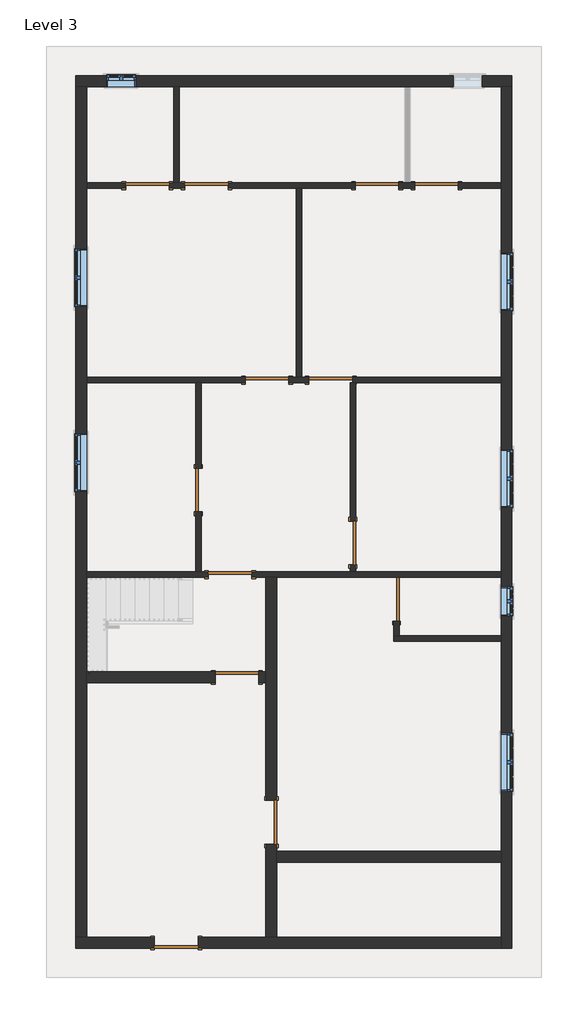
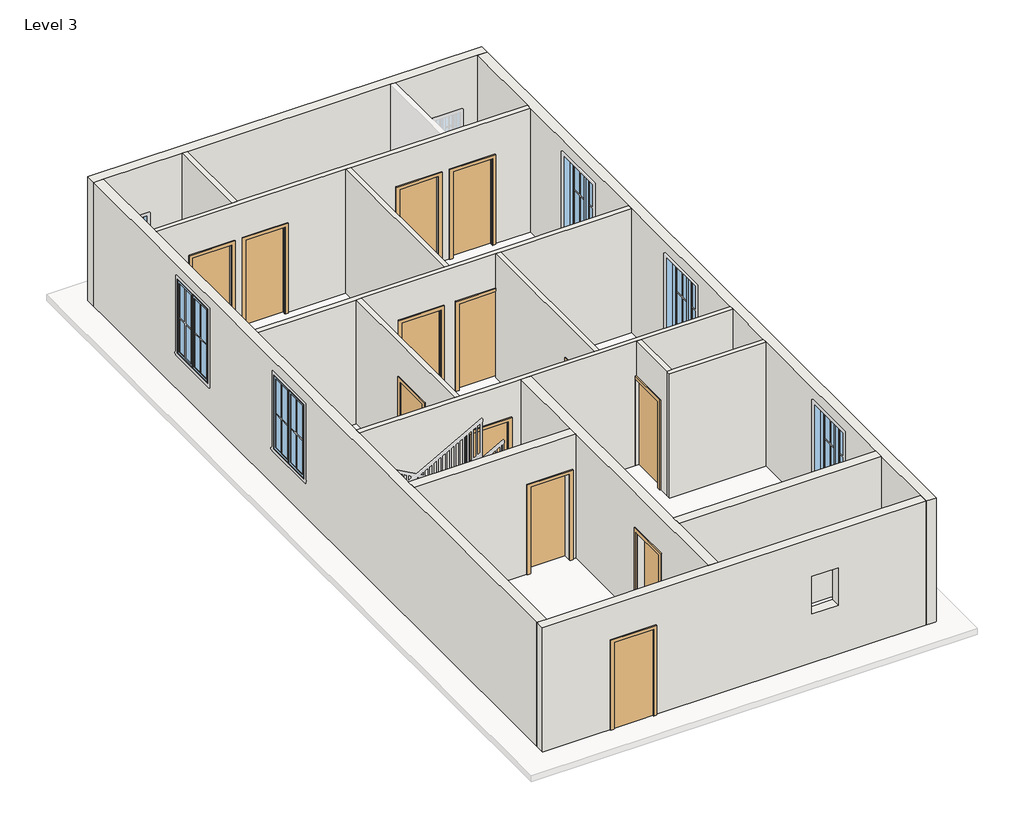
# One storey, part 1 of 3: 16 walls, 13 doors, 7 windows.
"""IFC4 building model written with IfcOpenShell, lengths in millimetres."""

from ifc_helpers import new_model, si_unit, frame, origin, place, context, project, spatial, polyline, outline, extrude, faceted_brep, transform, mapped, element, save
from components import door_305aa2a5, door_e5f9f3c4, door_0ca8825f, window_c417fced, window_6ca1769e

model = new_model("IFC4")

# Units and contexts
model_context = context("Model", 3, world=origin())
ifc_project = project(units=[si_unit("LENGTHUNIT", "METRE", prefix="MILLI")], contexts=[model_context])

# Site, building, storey
site = spatial("IfcSite", under=ifc_project)
building = spatial("IfcBuilding", under=site)
storey = spatial("IfcBuildingStorey", under=building, Name="Level 3", Elevation=6096.0)

# Doors
placement = place(None, origin())
door_shape = door_305aa2a5(model_context)
element("IfcDoor", 1, ObjectType="Single-Flush : 36\" x 84\"", at=placement, inside=storey, context=model_context, shape_type="MappedRepresentation", body=[
    mapped(door_shape, transform((4013.2, 11918.95, 6096.0), x_axis=(-1.0, 0.0, 0.0), y_axis=(0.0, -1.0, 0.0), z_axis=(0.0, 0.0, 1.0))),
])
element("IfcDoor", 2, ObjectType="Single-Flush : 36\" x 84\"", at=placement, inside=storey, context=model_context, shape_type="MappedRepresentation", body=[
    mapped(door_shape, transform((8832.85, 11918.95, 6096.0), x_axis=(-1.0, 0.0, 0.0), y_axis=(0.0, -1.0, 0.0), z_axis=(0.0, 0.0, 1.0))),
])
element("IfcDoor", 3, ObjectType="Single-Flush : 36\" x 84\"", at=placement, inside=storey, context=model_context, shape_type="MappedRepresentation", body=[
    mapped(door_shape, transform((6616.7, 7842.25, 6096.0), x_axis=(-1.0, 0.0, 0.0), y_axis=(0.0, -1.0, 0.0), z_axis=(0.0, 0.0, 1.0))),
])
element("IfcDoor", 4, ObjectType="Single-Flush : 36\" x 84\"", at=placement, inside=storey, context=model_context, shape_type="MappedRepresentation", body=[
    mapped(door_shape, transform((3841.75, 5537.2, 6096.0), x_axis=(0.0, -1.0, 0.0), y_axis=(1.0, 0.0, 0.0), z_axis=(0.0, 0.0, 1.0))),
])
door_2_shape = door_e5f9f3c4(model_context)
element("IfcDoor", 5, ObjectType="Single-Flush : 36\" x 84\"", at=placement, inside=storey, context=model_context, shape_type="MappedRepresentation", body=[
    mapped(door_2_shape, transform((2774.95, 11918.95, 6096.0), x_axis=(1.0, 0.0, 0.0), y_axis=(0.0, 1.0, 0.0), z_axis=(0.0, 0.0, 1.0))),
])
element("IfcDoor", 6, ObjectType="Single-Flush : 36\" x 84\"", at=placement, inside=storey, context=model_context, shape_type="MappedRepresentation", body=[
    mapped(door_2_shape, transform((7588.25, 11918.95, 6096.0), x_axis=(1.0, 0.0, 0.0), y_axis=(0.0, 1.0, 0.0), z_axis=(0.0, 0.0, 1.0))),
])
element("IfcDoor", 7, ObjectType="Single-Flush : 36\" x 84\"", at=placement, inside=storey, context=model_context, shape_type="MappedRepresentation", body=[
    mapped(door_2_shape, transform((5283.2, 7842.25, 6096.0), x_axis=(1.0, 0.0, 0.0), y_axis=(0.0, 1.0, 0.0), z_axis=(0.0, 0.0, 1.0))),
])
element("IfcDoor", 8, ObjectType="Single-Flush : 36\" x 84\"", at=placement, inside=storey, context=model_context, shape_type="MappedRepresentation", body=[
    mapped(door_2_shape, transform((4508.5, 3765.55, 6096.0), x_axis=(1.0, 0.0, 0.0), y_axis=(0.0, 1.0, 0.0), z_axis=(0.0, 0.0, 1.0))),
])
element("IfcDoor", 9, ObjectType="Single-Flush : 36\" x 84\"", at=placement, inside=storey, context=model_context, shape_type="MappedRepresentation", body=[
    mapped(door_2_shape, transform((7080.25, 4432.3, 6096.0), x_axis=(0.0, -1.0, 0.0), y_axis=(1.0, 0.0, 0.0), z_axis=(0.0, 0.0, 1.0))),
])
element("IfcDoor", 10, ObjectType="Single-Flush : 36\" x 84\"", at=placement, inside=storey, context=model_context, shape_type="MappedRepresentation", body=[
    mapped(door_2_shape, transform((7994.65, 3251.2, 6096.0), x_axis=(0.0, -1.0, 0.0), y_axis=(1.0, 0.0, 0.0), z_axis=(0.0, 0.0, 1.0))),
])
door_3_shape = door_0ca8825f(model_context)
element("IfcDoor", 11, ObjectType="Single-Flush : 36\" x 84\"", at=placement, inside=storey, context=model_context, shape_type="MappedRepresentation", body=[
    mapped(door_3_shape, transform((4648.2, 1612.9, 6096.0), x_axis=(1.0, 0.0, 0.0), y_axis=(0.0, 1.0, 0.0), z_axis=(0.0, 0.0, 1.0))),
])
element("IfcDoor", 12, ObjectType="Single-Flush : 36\" x 84\"", at=placement, inside=storey, context=model_context, shape_type="MappedRepresentation", body=[
    mapped(door_3_shape, transform((5372.1, -1422.4, 6096.0), x_axis=(0.0, -1.0, 0.0), y_axis=(1.0, 0.0, 0.0), z_axis=(0.0, 0.0, 1.0))),
])
element("IfcDoor", 13, ObjectType="Single-Flush : 36\" x 84\"", at=placement, inside=storey, context=model_context, shape_type="MappedRepresentation", body=[
    mapped(door_3_shape, transform((3378.2, -3949.7, 6096.0), x_axis=(-1.0, 0.0, 0.0), y_axis=(0.0, -1.0, 0.0), z_axis=(0.0, 0.0, 1.0))),
])

# Walls
element("IfcWall", 14, ObjectType="Generic - 5\"", at=placement, inside=storey, context=model_context, shape_type="Brep", body=[
    faceted_brep([(8045.45, 11861.8, 6096.0), (8375.65, 11861.8, 6096.0), (8375.65, 11861.8, 8229.6), (9290.05, 11861.8, 8229.6), (9290.05, 11861.8, 6096.0), (10185.4, 11861.8, 6096.0), (10185.4, 11861.8, 9144.0), (6007.1, 11861.8, 9144.0), (5892.8, 11861.8, 9144.0), (1498.6, 11861.8, 9144.0), (1498.6, 11861.8, 6096.0), (2317.75, 11861.8, 6096.0), (2317.75, 11861.8, 8229.6), (3232.15, 11861.8, 8229.6), (3232.15, 11861.8, 6096.0), (3556.0, 11861.8, 6096.0), (3556.0, 11861.8, 8229.6), (4470.4, 11861.8, 8229.6), (4470.4, 11861.8, 6096.0), (5892.8, 11861.8, 6096.0), (6007.1, 11861.8, 6096.0), (7131.05, 11861.8, 6096.0), (7131.05, 11861.8, 8229.6), (8045.45, 11861.8, 8229.6), (8375.65, 11976.1, 8229.6), (8375.65, 11976.1, 6096.0), (8280.4, 11976.1, 6096.0), (8166.1, 11976.1, 6096.0), (8045.45, 11976.1, 6096.0), (8045.45, 11976.1, 8229.6), (7131.05, 11976.1, 8229.6), (7131.05, 11976.1, 6096.0), (4470.4, 11976.1, 6096.0), (4470.4, 11976.1, 8229.6), (3556.0, 11976.1, 8229.6), (3556.0, 11976.1, 6096.0), (3441.7, 11976.1, 6096.0), (3327.4, 11976.1, 6096.0), (3232.15, 11976.1, 6096.0), (3232.15, 11976.1, 8229.6), (2317.75, 11976.1, 8229.6), (2317.75, 11976.1, 6096.0), (1498.6, 11976.1, 6096.0), (1498.6, 11976.1, 9144.0), (3327.4, 11976.1, 9144.0), (3441.7, 11976.1, 9144.0), (8166.1, 11976.1, 9144.0), (8280.4, 11976.1, 9144.0), (10185.4, 11976.1, 9144.0), (10185.4, 11976.1, 6096.0), (9290.05, 11976.1, 6096.0), (9290.05, 11976.1, 8229.6)], [[[0, 1, 2, 3, 4, 5, 6, 7, 8, 9, 10, 11, 12, 13, 14, 15, 16, 17, 18, 19, 20, 21, 22, 23]], [[24, 25, 26, 27, 28, 29, 30, 31, 32, 33, 34, 35, 36, 37, 38, 39, 40, 41, 42, 43, 44, 45, 46, 47, 48, 49, 50, 51]], [[11, 10, 42, 41]], [[15, 14, 38, 37, 36, 35]], [[21, 20, 19, 18, 32, 31]], [[50, 49, 5, 4]], [[28, 27, 26, 25, 1, 0]], [[9, 8, 7, 6, 48, 47, 46, 45, 44, 43]], [[6, 5, 49, 48]], [[10, 9, 43, 42]], [[16, 15, 35, 34]], [[17, 16, 34, 33]], [[18, 17, 33, 32]], [[39, 38, 14, 13]], [[40, 39, 13, 12]], [[41, 40, 12, 11]], [[29, 28, 0, 23]], [[30, 29, 23, 22]], [[31, 30, 22, 21]], [[2, 1, 25, 24]], [[3, 2, 24, 51]], [[4, 3, 51, 50]]]),
])
element("IfcWall", 15, ObjectType="Generic - 5\"", at=placement, inside=storey, context=model_context, shape_type="Brep", body=[
    faceted_brep([(5740.4, 7785.1, 6096.0), (6159.5, 7785.1, 6096.0), (6159.5, 7785.1, 8229.6), (7073.9, 7785.1, 8229.6), (7073.9, 7785.1, 6096.0), (7137.4, 7785.1, 6096.0), (10185.4, 7785.1, 6096.0), (10185.4, 7785.1, 9144.0), (7137.4, 7785.1, 9144.0), (7023.1, 7785.1, 9144.0), (3898.9, 7785.1, 9144.0), (3784.6, 7785.1, 9144.0), (1498.6, 7785.1, 9144.0), (1498.6, 7785.1, 6096.0), (3784.6, 7785.1, 6096.0), (3898.9, 7785.1, 6096.0), (4826.0, 7785.1, 6096.0), (4826.0, 7785.1, 8229.6), (5740.4, 7785.1, 8229.6), (6159.5, 7899.4, 8229.6), (6159.5, 7899.4, 6096.0), (6007.1, 7899.4, 6096.0), (5892.8, 7899.4, 6096.0), (5740.4, 7899.4, 6096.0), (5740.4, 7899.4, 8229.6), (4826.0, 7899.4, 8229.6), (4826.0, 7899.4, 6096.0), (1498.6, 7899.4, 6096.0), (1498.6, 7899.4, 9144.0), (5892.8, 7899.4, 9144.0), (6007.1, 7899.4, 9144.0), (10185.4, 7899.4, 9144.0), (10185.4, 7899.4, 6096.0), (7073.9, 7899.4, 6096.0), (7073.9, 7899.4, 8229.6)], [[[0, 1, 2, 3, 4, 5, 6, 7, 8, 9, 10, 11, 12, 13, 14, 15, 16, 17, 18]], [[19, 20, 21, 22, 23, 24, 25, 26, 27, 28, 29, 30, 31, 32, 33, 34]], [[16, 15, 14, 13, 27, 26]], [[33, 32, 6, 5, 4]], [[23, 22, 21, 20, 1, 0]], [[12, 11, 10, 9, 8, 7, 31, 30, 29, 28]], [[7, 6, 32, 31]], [[13, 12, 28, 27]], [[24, 23, 0, 18]], [[25, 24, 18, 17]], [[26, 25, 17, 16]], [[2, 1, 20, 19]], [[3, 2, 19, 34]], [[4, 3, 34, 33]]]),
])
element("IfcWall", 16, ObjectType="Generic - 5\"", at=placement, inside=storey, context=model_context, shape_type="SweptSolid", body=[
    extrude(outline(polyline([(5080.0, 8229.6), (5080.0, 6096.0), (3822.7, 6096.0), (3822.7, 9144.0), (7785.1, 9144.0), (7785.1, 6096.0), (5994.4, 6096.0), (5994.4, 8229.6), (5080.0, 8229.6)])), frame((3784.6, 0.0, 0.0), z_axis=(1.0, 0.0, 0.0), x_axis=(0.0, 1.0, 0.0)), (0.0, 0.0, 1.0), 114.3),
])
element("IfcWall", 17, ObjectType="Generic - 5\"", at=placement, inside=storey, context=model_context, shape_type="Brep", body=[
    faceted_brep([(4965.7, 3708.4, 8229.6), (4965.7, 3708.4, 6096.0), (5257.8, 3708.4, 6096.0), (5486.4, 3708.4, 6096.0), (10185.4, 3708.4, 6096.0), (10185.4, 3708.4, 9144.0), (8051.8, 3708.4, 9144.0), (7937.5, 3708.4, 9144.0), (5486.4, 3708.4, 9144.0), (5257.8, 3708.4, 9144.0), (1498.6, 3708.4, 9144.0), (1498.6, 3708.4, 6096.0), (4051.3, 3708.4, 6096.0), (4051.3, 3708.4, 8229.6), (10185.4, 3822.7, 6096.0), (7137.4, 3822.7, 6096.0), (7023.1, 3822.7, 6096.0), (4965.7, 3822.7, 6096.0), (4965.7, 3822.7, 8229.6), (4051.3, 3822.7, 8229.6), (4051.3, 3822.7, 6096.0), (3898.9, 3822.7, 6096.0), (3784.6, 3822.7, 6096.0), (1498.6, 3822.7, 6096.0), (1498.6, 3822.7, 9144.0), (3784.6, 3822.7, 9144.0), (3898.9, 3822.7, 9144.0), (7023.1, 3822.7, 9144.0), (7137.4, 3822.7, 9144.0), (10185.4, 3822.7, 9144.0)], [[[0, 1, 2, 3, 4, 5, 6, 7, 8, 9, 10, 11, 12, 13]], [[14, 15, 16, 17, 18, 19, 20, 21, 22, 23, 24, 25, 26, 27, 28, 29]], [[12, 11, 23, 22, 21, 20]], [[4, 3, 2, 1, 17, 16, 15, 14]], [[10, 9, 8, 7, 6, 5, 29, 28, 27, 26, 25, 24]], [[5, 4, 14, 29]], [[11, 10, 24, 23]], [[18, 17, 1, 0]], [[19, 18, 0, 13]], [[20, 19, 13, 12]]]),
])
element("IfcWall", 18, ObjectType="Generic - 5\"", at=placement, inside=storey, context=model_context, shape_type="Brep", body=[
    faceted_brep([(10185.4, 2489.2, 6096.0), (8051.8, 2489.2, 6096.0), (7937.5, 2489.2, 6096.0), (7937.5, 2489.2, 9144.0), (8051.8, 2489.2, 9144.0), (10185.4, 2489.2, 9144.0), (10185.4, 2374.9, 6096.0), (10185.4, 2374.9, 9144.0), (7937.5, 2374.9, 9144.0), (7937.5, 2374.9, 6096.0)], [[[0, 1, 2, 3, 4, 5]], [[6, 7, 8, 9]], [[2, 1, 0, 6, 9]], [[5, 4, 3, 8, 7]], [[0, 5, 7, 6]], [[3, 2, 9, 8]]]),
])
element("IfcWall", 19, ObjectType="Generic - 5\"", at=placement, inside=storey, context=model_context, shape_type="SweptSolid", body=[
    extrude(outline(polyline([(2489.2, 9144.0), (3708.4, 9144.0), (3708.4, 8229.6), (2794.0, 8229.6), (2794.0, 6096.0), (2489.2, 6096.0), (2489.2, 9144.0)])), frame((7937.5, 0.0, 0.0), z_axis=(1.0, 0.0, 0.0), x_axis=(0.0, 1.0, 0.0)), (0.0, 0.0, 1.0), 114.3),
])
element("IfcWall", 20, ObjectType="Generic - 5\"", at=placement, inside=storey, context=model_context, shape_type="Brep", body=[
    faceted_brep([(7023.1, 3975.1, 8229.6), (7023.1, 3975.1, 6096.0), (7023.1, 3822.7, 6096.0), (7023.1, 3822.7, 9144.0), (7023.1, 7785.1, 9144.0), (7023.1, 7785.1, 6096.0), (7023.1, 4889.5, 6096.0), (7023.1, 4889.5, 8229.6), (7137.4, 3822.7, 6096.0), (7137.4, 3975.1, 6096.0), (7137.4, 3975.1, 8229.6), (7137.4, 4889.5, 8229.6), (7137.4, 4889.5, 6096.0), (7137.4, 7785.1, 6096.0), (7137.4, 7785.1, 9144.0), (7137.4, 3822.7, 9144.0), (7073.9, 7785.1, 6096.0)], [[[0, 1, 2, 3, 4, 5, 6, 7]], [[8, 9, 10, 11, 12, 13, 14, 15]], [[6, 5, 16, 13, 12]], [[2, 1, 9, 8]], [[4, 3, 15, 14]], [[5, 4, 14, 13, 16]], [[3, 2, 8, 15]], [[10, 9, 1, 0]], [[11, 10, 0, 7]], [[12, 11, 7, 6]]]),
])
element("IfcWall", 21, ObjectType="Generic - 5\"", at=placement, inside=storey, context=model_context, shape_type="SweptSolid", body=[
    extrude(outline(polyline([(3327.4, 11976.1), (3327.4, 13995.4), (3441.7, 13995.4), (3441.7, 11976.1), (3327.4, 11976.1)])), frame((0.0, 0.0, 6096.0), z_axis=(0.0, 0.0, 1.0), x_axis=(1.0, 0.0, 0.0)), (0.0, 0.0, 1.0), 3048.0),
])
element("IfcWall", 22, ObjectType="Generic - 5\"", at=placement, inside=storey, context=model_context, shape_type="SweptSolid", body=[
    extrude(outline(polyline([(5892.8, 7899.4), (5892.8, 11861.8), (6007.1, 11861.8), (6007.1, 7899.4), (5892.8, 7899.4)])), frame((0.0, 0.0, 6096.0), z_axis=(0.0, 0.0, 1.0), x_axis=(1.0, 0.0, 0.0)), (0.0, 0.0, 1.0), 3048.0),
])
element("IfcWall", 23, ObjectType="Generic - 8\"", at=placement, inside=storey, context=model_context, shape_type="Brep", body=[
    faceted_brep([(1270.0, 13995.4, 6096.0), (1498.6, 13995.4, 6096.0), (3327.4, 13995.4, 6096.0), (3441.7, 13995.4, 6096.0), (8166.1, 13995.4, 6096.0), (8280.4, 13995.4, 6096.0), (10185.4, 13995.4, 6096.0), (10414.0, 13995.4, 6096.0), (10414.0, 13995.4, 9144.0), (10185.4, 13995.4, 9144.0), (8280.4, 13995.4, 9144.0), (8166.1, 13995.4, 9144.0), (3441.7, 13995.4, 9144.0), (3327.4, 13995.4, 9144.0), (1498.6, 13995.4, 9144.0), (1270.0, 13995.4, 9144.0), (9791.7, 13995.4, 7924.8), (9791.7, 13995.4, 7010.4), (9182.1, 13995.4, 7010.4), (9182.1, 13995.4, 7924.8), (2527.3, 13995.4, 7924.8), (2527.3, 13995.4, 7010.4), (1917.7, 13995.4, 7010.4), (1917.7, 13995.4, 7924.8), (1270.0, 14224.0, 6096.0), (1270.0, 14224.0, 9144.0), (10414.0, 14224.0, 9144.0), (10414.0, 14224.0, 6096.0), (9791.7, 14224.0, 7924.8), (9182.1, 14224.0, 7924.8), (9182.1, 14224.0, 7010.4), (9791.7, 14224.0, 7010.4), (2527.3, 14224.0, 7924.8), (1917.7, 14224.0, 7924.8), (1917.7, 14224.0, 7010.4), (2527.3, 14224.0, 7010.4)], [[[0, 1, 2, 3, 4, 5, 6, 7, 8, 9, 10, 11, 12, 13, 14, 15], [16, 17, 18, 19], [20, 21, 22, 23]], [[24, 25, 26, 27], [28, 29, 30, 31], [32, 33, 34, 35]], [[7, 6, 5, 4, 3, 2, 1, 0, 24, 27]], [[15, 14, 13, 12, 11, 10, 9, 8, 26, 25]], [[8, 7, 27, 26]], [[0, 15, 25, 24]], [[17, 16, 28, 31]], [[18, 17, 31, 30]], [[19, 18, 30, 29]], [[16, 19, 29, 28]], [[21, 20, 32, 35]], [[22, 21, 35, 34]], [[23, 22, 34, 33]], [[20, 23, 33, 32]]]),
])
element("IfcWall", 24, ObjectType="Generic - 8\"", at=placement, inside=storey, context=model_context, shape_type="Brep", body=[
    faceted_brep([(10185.4, 13995.4, 6096.0), (10185.4, 11976.1, 6096.0), (10185.4, 11861.8, 6096.0), (10185.4, 7899.4, 6096.0), (10185.4, 7785.1, 6096.0), (10185.4, 3822.7, 6096.0), (10185.4, 3708.4, 6096.0), (10185.4, 2489.2, 6096.0), (10185.4, 2374.9, 6096.0), (10185.4, -2032.0, 6096.0), (10185.4, -2260.6, 6096.0), (10185.4, -3835.4, 6096.0), (10185.4, -4064.0, 6096.0), (10185.4, -4064.0, 9144.0), (10185.4, -3835.4, 9144.0), (10185.4, -2260.6, 9144.0), (10185.4, -2032.0, 9144.0), (10185.4, 2374.9, 9144.0), (10185.4, 2489.2, 9144.0), (10185.4, 3708.4, 9144.0), (10185.4, 3822.7, 9144.0), (10185.4, 7785.1, 9144.0), (10185.4, 7899.4, 9144.0), (10185.4, 11861.8, 9144.0), (10185.4, 11976.1, 9144.0), (10185.4, 13995.4, 9144.0), (10185.4, 9296.4, 8839.2), (10185.4, 9296.4, 7010.4), (10185.4, 10515.6, 7010.4), (10185.4, 10515.6, 8839.2), (10185.4, 5168.9, 8839.2), (10185.4, 5168.9, 7010.4), (10185.4, 6388.1, 7010.4), (10185.4, 6388.1, 8839.2), (10185.4, -774.7, 8839.2), (10185.4, -774.7, 7010.4), (10185.4, 444.5, 7010.4), (10185.4, 444.5, 8839.2), (10185.4, 2901.95, 7924.8), (10185.4, 2901.95, 7010.4), (10185.4, 3511.55, 7010.4), (10185.4, 3511.55, 7924.8), (10414.0, 13995.4, 6096.0), (10414.0, 13995.4, 9144.0), (10414.0, -4064.0, 9144.0), (10414.0, -4064.0, 6096.0), (10414.0, 9296.4, 8839.2), (10414.0, 10515.6, 8839.2), (10414.0, 10515.6, 7010.4), (10414.0, 9296.4, 7010.4), (10414.0, 5168.9, 8839.2), (10414.0, 6388.1, 8839.2), (10414.0, 6388.1, 7010.4), (10414.0, 5168.9, 7010.4), (10414.0, -774.7, 8839.2), (10414.0, 444.5, 8839.2), (10414.0, 444.5, 7010.4), (10414.0, -774.7, 7010.4), (10414.0, 2901.95, 7924.8), (10414.0, 3511.55, 7924.8), (10414.0, 3511.55, 7010.4), (10414.0, 2901.95, 7010.4)], [[[0, 1, 2, 3, 4, 5, 6, 7, 8, 9, 10, 11, 12, 13, 14, 15, 16, 17, 18, 19, 20, 21, 22, 23, 24, 25], [26, 27, 28, 29], [30, 31, 32, 33], [34, 35, 36, 37], [38, 39, 40, 41]], [[42, 43, 44, 45], [46, 47, 48, 49], [50, 51, 52, 53], [54, 55, 56, 57], [58, 59, 60, 61]], [[12, 11, 10, 9, 8, 7, 6, 5, 4, 3, 2, 1, 0, 42, 45]], [[25, 24, 23, 22, 21, 20, 19, 18, 17, 16, 15, 14, 13, 44, 43]], [[0, 25, 43, 42]], [[13, 12, 45, 44]], [[27, 26, 46, 49]], [[28, 27, 49, 48]], [[29, 28, 48, 47]], [[26, 29, 47, 46]], [[31, 30, 50, 53]], [[32, 31, 53, 52]], [[33, 32, 52, 51]], [[30, 33, 51, 50]], [[35, 34, 54, 57]], [[36, 35, 57, 56]], [[37, 36, 56, 55]], [[34, 37, 55, 54]], [[39, 38, 58, 61]], [[40, 39, 61, 60]], [[41, 40, 60, 59]], [[38, 41, 59, 58]]]),
])
element("IfcWall", 25, ObjectType="Generic - 8\"", at=placement, inside=storey, context=model_context, shape_type="Brep", body=[
    faceted_brep([(2921.0, -3835.4, 8229.6), (2921.0, -3835.4, 6096.0), (1498.6, -3835.4, 6096.0), (1270.0, -3835.4, 6096.0), (1270.0, -3835.4, 9144.0), (1498.6, -3835.4, 9144.0), (5257.8, -3835.4, 9144.0), (5486.4, -3835.4, 9144.0), (10185.4, -3835.4, 9144.0), (10185.4, -3835.4, 6096.0), (5486.4, -3835.4, 6096.0), (5257.8, -3835.4, 6096.0), (3835.4, -3835.4, 6096.0), (3835.4, -3835.4, 8229.6), (7531.1, -3835.4, 8215.2257161), (7531.1, -3835.4, 7300.8257161), (8140.7, -3835.4, 7300.8257161), (8140.7, -3835.4, 8215.2257161), (1270.0, -4064.0, 6096.0), (2921.0, -4064.0, 6096.0), (2921.0, -4064.0, 8229.6), (3835.4, -4064.0, 8229.6), (3835.4, -4064.0, 6096.0), (10185.4, -4064.0, 6096.0), (10185.4, -4064.0, 9144.0), (1270.0, -4064.0, 9144.0), (7531.1, -4064.0, 8215.2257161), (8140.7, -4064.0, 8215.2257161), (8140.7, -4064.0, 7300.8257161), (7531.1, -4064.0, 7300.8257161)], [[[0, 1, 2, 3, 4, 5, 6, 7, 8, 9, 10, 11, 12, 13], [14, 15, 16, 17]], [[18, 19, 20, 21, 22, 23, 24, 25], [26, 27, 28, 29]], [[3, 2, 1, 19, 18]], [[12, 11, 10, 9, 23, 22]], [[8, 7, 6, 5, 4, 25, 24]], [[9, 8, 24, 23]], [[4, 3, 18, 25]], [[20, 19, 1, 0]], [[21, 20, 0, 13]], [[22, 21, 13, 12]], [[15, 14, 26, 29]], [[16, 15, 29, 28]], [[17, 16, 28, 27]], [[14, 17, 27, 26]]]),
])
element("IfcWall", 26, ObjectType="Generic - 8\"", at=placement, inside=storey, context=model_context, shape_type="Brep", body=[
    faceted_brep([(1498.6, -3835.4, 6096.0), (1498.6, 1498.6, 6096.0), (1498.6, 1727.2, 6096.0), (1498.6, 3708.4, 6096.0), (1498.6, 3822.7, 6096.0), (1498.6, 7785.1, 6096.0), (1498.6, 7899.4, 6096.0), (1498.6, 11861.8, 6096.0), (1498.6, 11976.1, 6096.0), (1498.6, 13995.4, 6096.0), (1498.6, 13995.4, 9144.0), (1498.6, 11976.1, 9144.0), (1498.6, 11861.8, 9144.0), (1498.6, 7899.4, 9144.0), (1498.6, 7785.1, 9144.0), (1498.6, 3822.7, 9144.0), (1498.6, 3708.4, 9144.0), (1498.6, 1727.2, 9144.0), (1498.6, 1498.6, 9144.0), (1498.6, -3835.4, 9144.0), (1498.6, 6724.65, 8839.2), (1498.6, 6724.65, 7010.4), (1498.6, 5505.45, 7010.4), (1498.6, 5505.45, 8839.2), (1498.6, 10598.15, 8839.2), (1498.6, 10598.15, 7010.4), (1498.6, 9378.95, 7010.4), (1498.6, 9378.95, 8839.2), (1270.0, -3835.4, 6096.0), (1270.0, -3835.4, 9144.0), (1270.0, 13995.4, 9144.0), (1270.0, 13995.4, 6096.0), (1270.0, 6724.65, 8839.2), (1270.0, 5505.45, 8839.2), (1270.0, 5505.45, 7010.4), (1270.0, 6724.65, 7010.4), (1270.0, 10598.15, 8839.2), (1270.0, 9378.95, 8839.2), (1270.0, 9378.95, 7010.4), (1270.0, 10598.15, 7010.4)], [[[0, 1, 2, 3, 4, 5, 6, 7, 8, 9, 10, 11, 12, 13, 14, 15, 16, 17, 18, 19], [20, 21, 22, 23], [24, 25, 26, 27]], [[28, 29, 30, 31], [32, 33, 34, 35], [36, 37, 38, 39]], [[9, 8, 7, 6, 5, 4, 3, 2, 1, 0, 28, 31]], [[19, 18, 17, 16, 15, 14, 13, 12, 11, 10, 30, 29]], [[10, 9, 31, 30]], [[21, 20, 32, 35]], [[22, 21, 35, 34]], [[23, 22, 34, 33]], [[20, 23, 33, 32]], [[25, 24, 36, 39]], [[26, 25, 39, 38]], [[27, 26, 38, 37]], [[24, 27, 37, 36]], [[0, 19, 29, 28]]]),
])
element("IfcWall", 27, ObjectType="Generic - 8\"", at=placement, inside=storey, context=model_context, shape_type="SweptSolid", body=[
    extrude(outline(polyline([(8229.6, 5105.4), (6096.0, 5105.4), (6096.0, 5257.8), (9144.0, 5257.8), (9144.0, 1498.6), (6096.0, 1498.6), (6096.0, 4191.0), (8229.6, 4191.0), (8229.6, 5105.4)])), frame((0.0, 1498.6, 0.0), z_axis=(0.0, 1.0, 0.0), x_axis=(0.0, 0.0, 1.0)), (0.0, 0.0, 1.0), 228.6),
])
element("IfcWall", 28, ObjectType="Generic - 8\"", at=placement, inside=storey, context=model_context, shape_type="Brep", body=[
    faceted_brep([(5257.8, -1879.6, 8229.6), (5257.8, -1879.6, 6096.0), (5257.8, -3835.4, 6096.0), (5257.8, -3835.4, 9144.0), (5257.8, 1498.6, 9144.0), (5257.8, 1727.2, 9144.0), (5257.8, 3708.4, 9144.0), (5257.8, 3708.4, 6096.0), (5257.8, 1727.2, 6096.0), (5257.8, 1498.6, 6096.0), (5257.8, -965.2, 6096.0), (5257.8, -965.2, 8229.6), (5486.4, -3835.4, 6096.0), (5486.4, -2260.6, 6096.0), (5486.4, -2032.0, 6096.0), (5486.4, -1879.6, 6096.0), (5486.4, -1879.6, 8229.6), (5486.4, -965.2, 8229.6), (5486.4, -965.2, 6096.0), (5486.4, 3708.4, 6096.0), (5486.4, 3708.4, 9144.0), (5486.4, -2032.0, 9144.0), (5486.4, -2260.6, 9144.0), (5486.4, -3835.4, 9144.0)], [[[0, 1, 2, 3, 4, 5, 6, 7, 8, 9, 10, 11]], [[12, 13, 14, 15, 16, 17, 18, 19, 20, 21, 22, 23]], [[2, 1, 15, 14, 13, 12]], [[10, 9, 8, 7, 19, 18]], [[6, 5, 4, 3, 23, 22, 21, 20]], [[3, 2, 12, 23]], [[7, 6, 20, 19]], [[16, 15, 1, 0]], [[17, 16, 0, 11]], [[18, 17, 11, 10]]]),
])
element("IfcWall", 29, ObjectType="Generic - 8\"", at=placement, inside=storey, context=model_context, shape_type="SweptSolid", body=[
    extrude(outline(polyline([(10185.4, -2260.6), (5486.4, -2260.6), (5486.4, -2032.0), (10185.4, -2032.0), (10185.4, -2260.6)])), frame((0.0, 0.0, 6096.0), z_axis=(0.0, 0.0, 1.0), x_axis=(1.0, 0.0, 0.0)), (0.0, 0.0, 1.0), 3048.0),
])

# Windows
window_shape = window_c417fced(model_context)
element("IfcWindow", 30, ObjectType="Window-Casement-Double : 24\" x 36\"", at=placement, inside=storey, context=model_context, shape_type="MappedRepresentation", body=[
    mapped(window_shape, transform((10299.7, 3206.75, 6096.0), x_axis=(0.0, -1.0, 0.0), y_axis=(1.0, 0.0, 0.0), z_axis=(0.0, 0.0, 1.0))),
])
element("IfcWindow", 31, ObjectType="Window-Casement-Double : 24\" x 36\"", at=placement, inside=storey, context=model_context, shape_type="MappedRepresentation", body=[
    mapped(window_shape, transform((2222.5, 14109.7, 6096.0), x_axis=(1.0, 0.0, 0.0), y_axis=(0.0, 1.0, 0.0), z_axis=(0.0, 0.0, 1.0))),
])
window_2_shape = window_6ca1769e(model_context)
element("IfcWindow", 32, ObjectType="Window-Casement-Double : 48\" x 72\"", at=placement, inside=storey, context=model_context, shape_type="MappedRepresentation", body=[
    mapped(window_2_shape, transform((1384.3, 6115.05, 6096.0), x_axis=(0.0, 1.0, 0.0), y_axis=(-1.0, 0.0, 0.0), z_axis=(0.0, 0.0, 1.0))),
])
element("IfcWindow", 33, ObjectType="Window-Casement-Double : 48\" x 72\"", at=placement, inside=storey, context=model_context, shape_type="MappedRepresentation", body=[
    mapped(window_2_shape, transform((1384.3, 9988.55, 6096.0), x_axis=(0.0, 1.0, 0.0), y_axis=(-1.0, 0.0, 0.0), z_axis=(0.0, 0.0, 1.0))),
])
element("IfcWindow", 34, ObjectType="Window-Casement-Double : 48\" x 72\"", at=placement, inside=storey, context=model_context, shape_type="MappedRepresentation", body=[
    mapped(window_2_shape, transform((10299.7, 9906.0, 6096.0), x_axis=(0.0, -1.0, 0.0), y_axis=(1.0, 0.0, 0.0), z_axis=(0.0, 0.0, 1.0))),
])
element("IfcWindow", 35, ObjectType="Window-Casement-Double : 48\" x 72\"", at=placement, inside=storey, context=model_context, shape_type="MappedRepresentation", body=[
    mapped(window_2_shape, transform((10299.7, 5778.5, 6096.0), x_axis=(0.0, -1.0, 0.0), y_axis=(1.0, 0.0, 0.0), z_axis=(0.0, 0.0, 1.0))),
])
element("IfcWindow", 36, ObjectType="Window-Casement-Double : 48\" x 72\"", at=placement, inside=storey, context=model_context, shape_type="MappedRepresentation", body=[
    mapped(window_2_shape, transform((10299.7, -165.1, 6096.0), x_axis=(0.0, -1.0, 0.0), y_axis=(1.0, 0.0, 0.0), z_axis=(0.0, 0.0, 1.0))),
])

save(model, "model.ifc")

# Revit data of these elements
# Type "Single-Flush : 36\" x 84\""
#   Type Mark = "1"
#   Construction Type Id = "MDOOR"
#   Assembly Code = "C1020"
#   Analytic Construction = "Metal"
#   Thickness = 0' - 2"
#   Heat Transfer Coefficient (U) = 0.651978 BTU/(h·ft²·°F)
#   Height = 7' - 0"
#   Trim Projection Ext = 0' - 1"
#   Trim Projection Int = 0' - 1"
#   Trim Width = 0' - 3"
#   Width = 3' - 0"
#   Define Thermal Properties by = 1
#   Define Thermal Properties by = 1
#   Door Material = Door - Panel
#   Frame Material = Door - Frame
#   Visual Light Transmittance = 0
#   Solar Heat Gain Coefficient = 0
#   Function = (empty or 0)
#   Wall Closure = (empty or 0)
# Type "Generic - 5\""
#   Assembly Code = "B2010"
#   Layers, outside or top first: 0' - 4 1/2" no material (function 1)
# Type "Generic - 8\""
#   Assembly Code = "B2010"
#   Layers, outside or top first: 0' - 9" "Parking Stripe" (function 1)
# Type "Window-Casement-Double : 24\" x 36\""
#   Type Mark = "14"
#   Fire Rating = "0.5h"
#   Assembly Code = "B2020100"
#   Analytic Construction = "Double glazing - domestic"
#   Frame Extension [instance default] = 0' - 0 1/4"
#   Window Inset [instance default] = 0' - 0"
#   Wall Thickness [instance default] = 0' - 6"
#   Interior Wall Closure [instance default] = 0' - 2 1/4"
#   Half Width = 1' - 0"
#   Visual Light Transmittance = 0.81
#   Thermal Resistance (R) = 1.8146 (h·ft²·°F)/BTU
#   Solar Heat Gain Coefficient = 0.76
#   Rough Width = 2' - 0 1/2"
#   Rough Height = 3' - 0 1/2"
#   Height = 3' - 0"
#   Heat Transfer Coefficient (U) = 0.5511 BTU/(h·ft²·°F)
#   Exterior Wall Closure [instance default] = 0' - 1 1/4"
#   Extension Jamb [instance default] = 0' - 2 1/4"
#   Default Sill Height = 3' - 0"
#   Width = 2' - 0"
#   Define Thermal Properties by = 0
#   Muntin Visibility = yes
#   Interior Trim Visibility [instance default] = yes
#   Exterior Trim Visibility [instance default] = yes
#   Extension Jamb Visibility [instance default] = yes
#   Interior Trim Material = Wood - Stained
#   Muntin Pattern = Muntin Pattern_2x2 : Muntin Pattern_2x2
#   Interior Trim = Trim-Window-Interior-Flat : Picture Frame
#   Interior Frame Material = Wood - Stained
#   Glass Panel Material = Glass
#   Exterior Trim Material = Clad - White
#   Exterior Trim = Trim-Window-Exterior-Flat : with Sill
#   Exterior Frame Material = Clad - White
#   Wall Closure = (empty or 0)
# Type "Window-Casement-Double : 48\" x 72\""
#   Type Mark = "17"
#   Fire Rating = "0.5h"
#   Assembly Code = "B2020100"
#   Analytic Construction = "Double glazing - domestic"
#   Frame Extension [instance default] = 0' - 0 1/4"
#   Window Inset [instance default] = 0' - 0"
#   Wall Thickness [instance default] = 0' - 6"
#   Interior Wall Closure [instance default] = 0' - 2 1/4"
#   Half Width = 2' - 0"
#   Visual Light Transmittance = 0.81
#   Thermal Resistance (R) = 1.8146 (h·ft²·°F)/BTU
#   Solar Heat Gain Coefficient = 0.76
#   Rough Width = 4' - 0 1/2"
#   Rough Height = 6' - 0 1/2"
#   Height = 6' - 0"
#   Heat Transfer Coefficient (U) = 0.5511 BTU/(h·ft²·°F)
#   Exterior Wall Closure [instance default] = 0' - 1 1/4"
#   Extension Jamb [instance default] = 0' - 2 1/4"
#   Default Sill Height = 3' - 0"
#   Width = 4' - 0"
#   Define Thermal Properties by = 0
#   Muntin Visibility = yes
#   Interior Trim Visibility [instance default] = yes
#   Exterior Trim Visibility [instance default] = yes
#   Extension Jamb Visibility [instance default] = yes
#   Interior Trim Material = Wood - Stained
#   Muntin Pattern = Muntin Pattern_2x2 : Muntin Pattern_2x2
#   Interior Trim = Trim-Window-Interior-Flat : Picture Frame
#   Interior Frame Material = Wood - Stained
#   Glass Panel Material = Glass
#   Exterior Trim Material = Clad - White
#   Exterior Trim = Trim-Window-Exterior-Flat : with Sill
#   Exterior Frame Material = Clad - White
#   Wall Closure = (empty or 0)
# Elements 1, 2, 3, 4, 5, 6, 7, 8, 9, 10, 11, 12, 13 (IfcDoor, "Single-Flush : 36\" x 84\"")
#   Phase Created = New Construction
#   Materials on its faces: "Door - Frame", "Door - Panel"
# Elements 14, 15, 16, 17, 18, 19, 20, 21, 22 (IfcWall, "Generic - 5\"")
#   Top Offset = 0' - 0"
#   Base Offset = 0' - 0"
#   wall height = 10' - 0"
#   Phase Created = New Construction
#   Base Constraint = Level 3
#   Top Constraint = Level 4
#   Materials on its faces: "Default Wall"
# Elements 23, 24, 25, 26, 27, 28, 29 (IfcWall, "Generic - 8\"")
#   Top Offset = 0' - 0"
#   Base Offset = 0' - 0"
#   Unconnected Height = 10' - 0"
#   wall height = 10' - 0"
#   Phase Created = New Construction
#   Base Constraint = Level 3
#   Materials on its faces: "Parking Stripe"
# Element 30 (IfcWindow, "Window-Casement-Double : 24\" x 36\"")
#   Mark = "22"
#   Window Inset = 0' - 0"
#   Interior Wall Closure = 0' - 2 1/4"
#   Frame Extension = 0' - 0 1/4"
#   Exterior Wall Closure = 0' - 1 1/4"
#   Interior Trim Visibility = yes
#   Exterior Trim Visibility = yes
#   Phase Created = New Construction
#   Materials on its faces: "Wood - Stained", "Glass", "Clad - White"
# Element 31 (IfcWindow, "Window-Casement-Double : 24\" x 36\"")
#   Mark = "24"
#   Window Inset = 0' - 0"
#   Interior Wall Closure = 0' - 2 1/4"
#   Frame Extension = 0' - 0 1/4"
#   Exterior Wall Closure = 0' - 1 1/4"
#   Interior Trim Visibility = yes
#   Exterior Trim Visibility = yes
#   Phase Created = New Construction
#   Materials on its faces: "Wood - Stained", "Glass", "Clad - White"
# Element 32 (IfcWindow, "Window-Casement-Double : 48\" x 72\"")
#   Mark = "17"
#   Window Inset = 0' - 0"
#   Interior Wall Closure = 0' - 2 1/4"
#   Frame Extension = 0' - 0 1/4"
#   Exterior Wall Closure = 0' - 1 1/4"
#   Interior Trim Visibility = yes
#   Exterior Trim Visibility = yes
#   Phase Created = New Construction
#   Materials on its faces: "Wood - Stained", "Glass", "Clad - White"
# Element 33 (IfcWindow, "Window-Casement-Double : 48\" x 72\"")
#   Mark = "18"
#   Window Inset = 0' - 0"
#   Interior Wall Closure = 0' - 2 1/4"
#   Frame Extension = 0' - 0 1/4"
#   Exterior Wall Closure = 0' - 1 1/4"
#   Interior Trim Visibility = yes
#   Exterior Trim Visibility = yes
#   Phase Created = New Construction
#   Materials on its faces: "Wood - Stained", "Glass", "Clad - White"
# Element 34 (IfcWindow, "Window-Casement-Double : 48\" x 72\"")
#   Mark = "19"
#   Window Inset = 0' - 0"
#   Interior Wall Closure = 0' - 2 1/4"
#   Frame Extension = 0' - 0 1/4"
#   Exterior Wall Closure = 0' - 1 1/4"
#   Interior Trim Visibility = yes
#   Exterior Trim Visibility = yes
#   Phase Created = New Construction
#   Materials on its faces: "Wood - Stained", "Glass", "Clad - White"
# Element 35 (IfcWindow, "Window-Casement-Double : 48\" x 72\"")
#   Mark = "20"
#   Window Inset = 0' - 0"
#   Interior Wall Closure = 0' - 2 1/4"
#   Frame Extension = 0' - 0 1/4"
#   Exterior Wall Closure = 0' - 1 1/4"
#   Interior Trim Visibility = yes
#   Exterior Trim Visibility = yes
#   Phase Created = New Construction
#   Materials on its faces: "Wood - Stained", "Glass", "Clad - White"
# Element 36 (IfcWindow, "Window-Casement-Double : 48\" x 72\"")
#   Mark = "21"
#   Window Inset = 0' - 0"
#   Interior Wall Closure = 0' - 2 1/4"
#   Frame Extension = 0' - 0 1/4"
#   Exterior Wall Closure = 0' - 1 1/4"
#   Interior Trim Visibility = yes
#   Exterior Trim Visibility = yes
#   Phase Created = New Construction
#   Materials on its faces: "Wood - Stained", "Glass", "Clad - White"
# Materials
#   "Door - Panel": class "Wood", colour RGB 210 159 95, transparency 0, Cost = 0
#   "Door - Frame": colour RGB 118 70 51, transparency 0, Cost = 0
#   "Parking Stripe": class "Paint", colour RGB 250 250 91, transparency 0, Cost = 0
#   "Wood - Stained": class "Wood", colour RGB 224 178 126, transparency 0, Cost = 0
#   "Glass": class "Glass", colour RGB 0 128 192, transparency 0.75, Description = "Soda Lime Glass", Cost = 0
#   "Clad - White": class "Wood", colour RGB 242 242 238, transparency 0, Cost = 0
#   "Default Wall": colour RGB 128 128 128, transparency 0, Cost = 0
